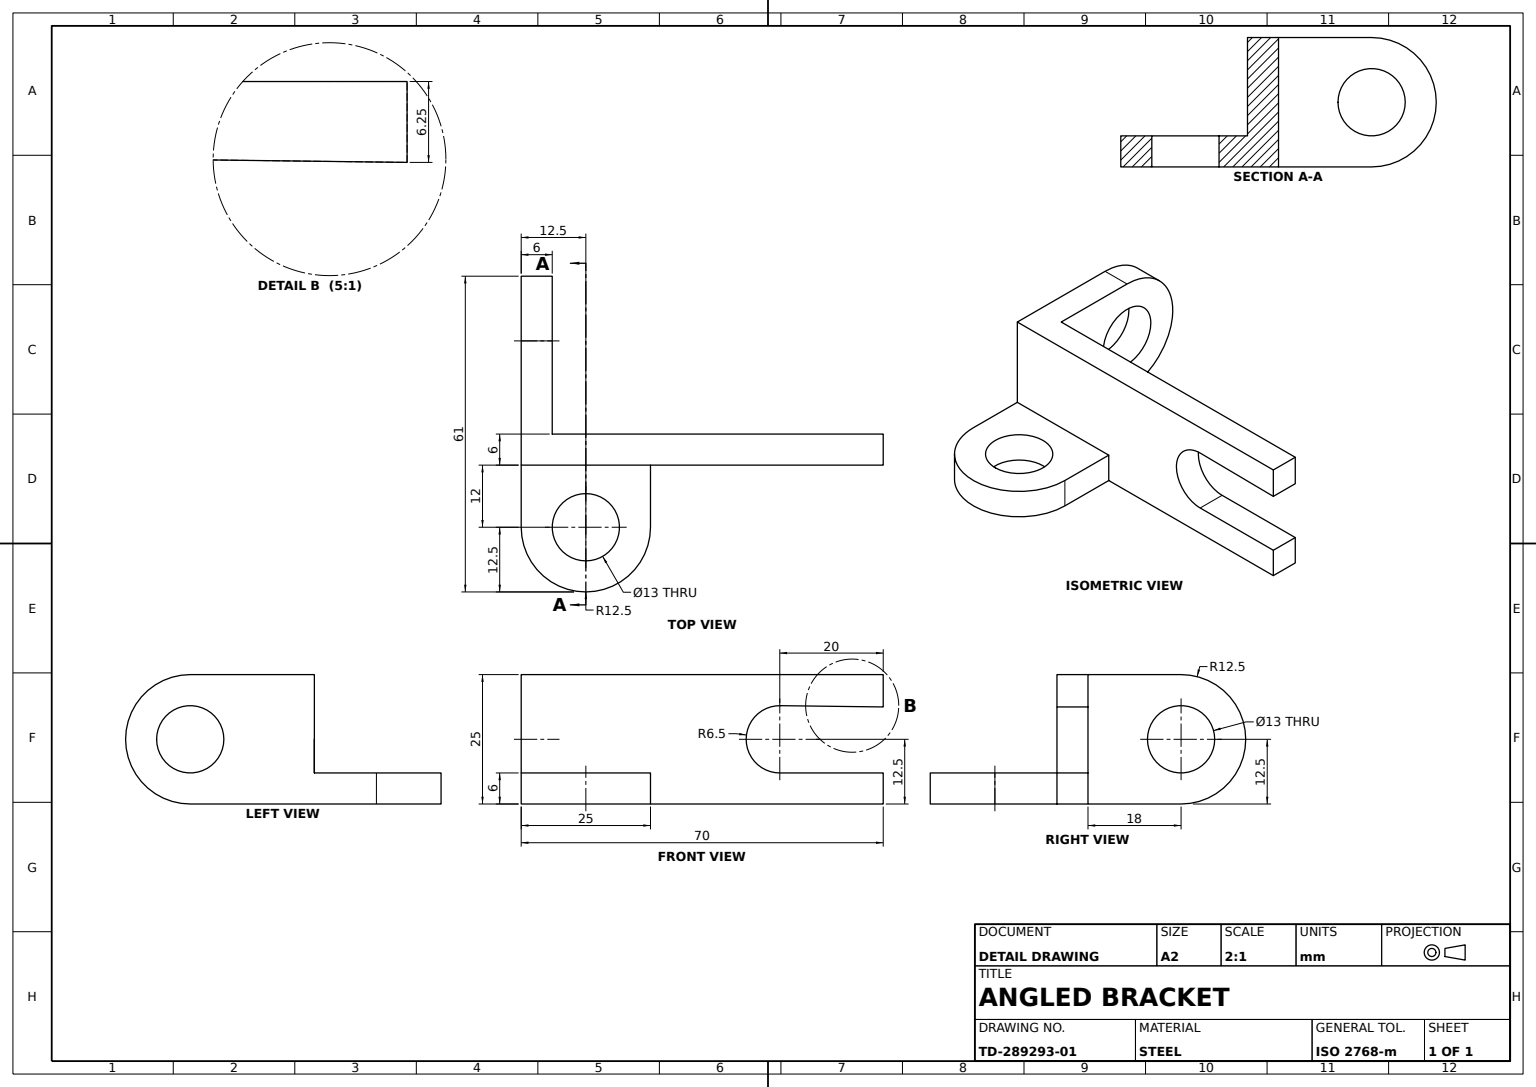
from build123d import *

# Parameters (mm, degrees)
SLOTTED_BRACKET_BODY_DEPTH = 6
LUG_A_SKETCH_R             = 6.5
MOUNTING_LUG_A_13_DEPTH    = 6
LUG_B_SKETCH_R             = 6.5
MOUNTING_LUG_B_13_DEPTH    = 6


with BuildPart() as part:
    # Bracket Profile Sketch → Slotted Bracket Body (new body)
    with BuildSketch(Plane.XY):
        with BuildLine():
            Line((-35.440613027, 25), (-35.440613027, 0))
            Line((-35.440613027, 0), (34.559386973, 0))
            Line((34.559386973, 0), (34.559386973, 6))
            Line((34.559386973, 6), (14.559386973, 6))
            ThreePointArc((14.559386973, 6), (8.059386973, 12.5), (14.559386973, 19))
            ThreePointArc((14.559386973, 19), (14.640630626, 18.999492247), (14.721861587, 18.997969067))
            Line((14.721861587, 18.997969067), (34.559386973, 18.75))
            Line((34.559386973, 18.75), (34.559386973, 25))
            Line((34.559386973, 25), (-35.440613027, 25))
        make_face()
    extrude(amount=SLOTTED_BRACKET_BODY_DEPTH)

    # Lug A Sketch → Mounting Lug A Ø13 (add)
    with BuildSketch(Plane.ZY.offset(35.440613027)):
        with BuildLine():
            Line((-18, 0), (6, 0))
            Line((6, 0), (6, 25))
            Line((6, 25), (-18, 25))
            ThreePointArc((-18, 25), (-30.5, 12.5), (-18, 0))
        make_face()
        with Locations((-18, 12.5)):
            Circle(LUG_A_SKETCH_R, mode=Mode.SUBTRACT)
    extrude(amount=-MOUNTING_LUG_A_13_DEPTH)

    # Lug B Sketch → Mounting Lug B Ø13 (add)
    with BuildSketch(Plane.XZ):
        with BuildLine():
            Line((-35.440613027, 18), (-35.440613027, 0))
            Line((-35.440613027, 0), (-10.440613027, 0))
            Line((-10.440613027, 0), (-10.440613027, 18))
            ThreePointArc((-10.440613027, 18), (-22.940613027, 30.5), (-35.440613027, 18))
        make_face()
        with Locations(Location((-22.940613027, 18, 0), (0, 0, 270))):
            Circle(LUG_B_SKETCH_R, mode=Mode.SUBTRACT)
    extrude(amount=-MOUNTING_LUG_B_13_DEPTH)


solid = part.part
